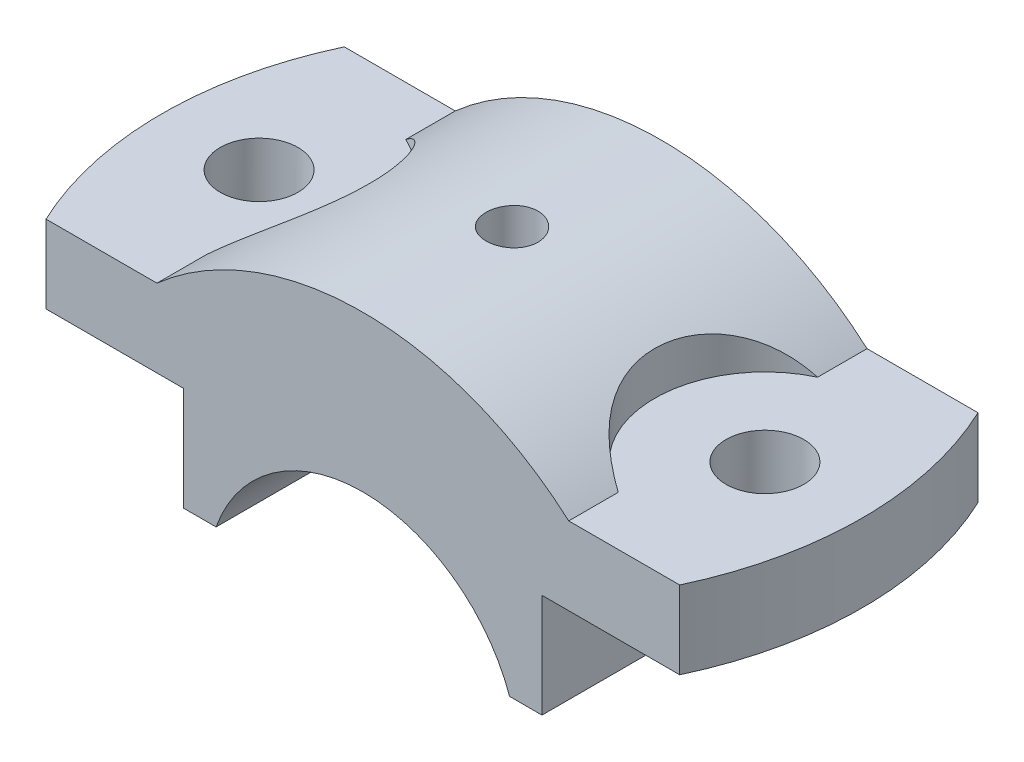
from build123d import *

# Parameters (mm, degrees)
CAP_BODY_DEPTH               = 23
BOLT_HOLES_12_D              = 12
SKETCH7_W                    = 17
SKETCH7_H                    = 36
HOLE_34_AT_2_COUNT           = 2
HOLE_34_AT_2_PITCH           = 78
LUBE_COUNTERBORE_SKETCH_8_R  = 4
LUBE_COUNTERBORE_8_DEPTH     = 16
LUBE_HOLE_SKETCH_6_R         = 3
LUBE_HOLE_6_DEPTH            = 72.028163461
SIDE_RELIEF_SKETCH_OUTSIDE_W = 134.804
SIDE_RELIEF_SKETCH_OUTSIDE_H = 72.804
SIDE_RELIEF_CUT_DEPTH        = 66.03076203


with BuildPart() as part:
    # Cap Profile Sketch → Cap Body (new, symmetric)
    with BuildSketch(Plane.XY):
        with BuildLine():
            Line((-22.627416998, 8), (-27.627416998, 8))
            Line((-27.627416998, 8), (-27.627416998, 24))
            Line((-27.627416998, 24), (-54, 24))
            Line((-54, 24), (-54, 36))
            Line((-54, 36), (-31.749015733, 36))
            ThreePointArc((-31.749015733, 36), (0, 48), (31.749015733, 36))
            Line((31.749015733, 36), (54, 36))
            Line((54, 36), (54, 24))
            Line((54, 24), (27.627416998, 24))
            Line((27.627416998, 24), (27.627416998, 8))
            Line((27.627416998, 8), (22.627416998, 8))
            ThreePointArc((22.627416998, 8), (0, 24), (-22.627416998, 8))
        make_face()
    extrude(amount=CAP_BODY_DEPTH, both=True)

    # Bolt Holes Ø12 (through all)
    with Locations(Plane(origin=(0, 36, 0), x_dir=(1, 0, 0), z_dir=(0, 1, 0))):
        with Locations((-39, 0), (39, 0)):
            Hole(BOLT_HOLES_12_D / 2)

    # Sketch7 → Hole Ø34 (revolve, cut)
    with BuildSketch(Plane(origin=(-39, 36, 0), x_dir=(0, 0, -1), z_dir=(1, 0, 0))):
        with Locations((8.5, 18)):
            Rectangle(SKETCH7_W, SKETCH7_H)
    hole_34 = revolve(axis=Axis((-39, 29.65, 0), (0, 1, 0)), mode=Mode.SUBTRACT)

    # Hole Ø34 at 2: Hole Ø34 ×2
    with Locations(*[(i * HOLE_34_AT_2_PITCH, 0, 0) for i in range(1, HOLE_34_AT_2_COUNT)]):
        add(hole_34, mode=Mode.SUBTRACT)

    # Lube Counterbore Sketch Ø8 → Lube Counterbore Ø8 (cut)
    with BuildSketch(Plane(origin=(0, 48, 0), x_dir=(1, 0, 0), z_dir=(0, 1, 0))):
        with Locations(Location((0, 0, 0), (0, 0, 270))):
            Circle(LUBE_COUNTERBORE_SKETCH_8_R)
    extrude(amount=-LUBE_COUNTERBORE_8_DEPTH, mode=Mode.SUBTRACT)

    # Lube Hole Sketch Ø6 → Lube Hole Ø6 (cut, through all)
    with BuildSketch(Plane(origin=(0, 48, 0), x_dir=(1, 0, 0), z_dir=(0, 1, 0))):
        with Locations(Location((0, 0, 0), (0, 0, 270))):
            Circle(LUBE_HOLE_SKETCH_6_R)
    extrude(amount=-LUBE_HOLE_6_DEPTH, mode=Mode.SUBTRACT)

    # Side Relief Sketch outside → Side Relief Cut (cut, through all)
    with BuildSketch(Plane(origin=(0, 36, 0), x_dir=(1, 0, 0), z_dir=(0, 1, 0))):
        Rectangle(SIDE_RELIEF_SKETCH_OUTSIDE_W, SIDE_RELIEF_SKETCH_OUTSIDE_H)
        with BuildLine():
            Line((-31.749015733, 23), (31.749015733, 23))
            Line((31.749015733, 23), (48.856934001, 23))
            ThreePointArc((48.856934001, 23), (54, 0), (48.856934001, -23))
            Line((48.856934001, -23), (31.749015733, -23))
            Line((31.749015733, -23), (-31.749015733, -23))
            Line((-31.749015733, -23), (-48.856934001, -23))
            ThreePointArc((-48.856934001, -23), (-54, 0), (-48.856934001, 23))
            Line((-48.856934001, 23), (-31.749015733, 23))
        make_face(mode=Mode.SUBTRACT)
    extrude(amount=-SIDE_RELIEF_CUT_DEPTH, mode=Mode.SUBTRACT)


solid = part.part
